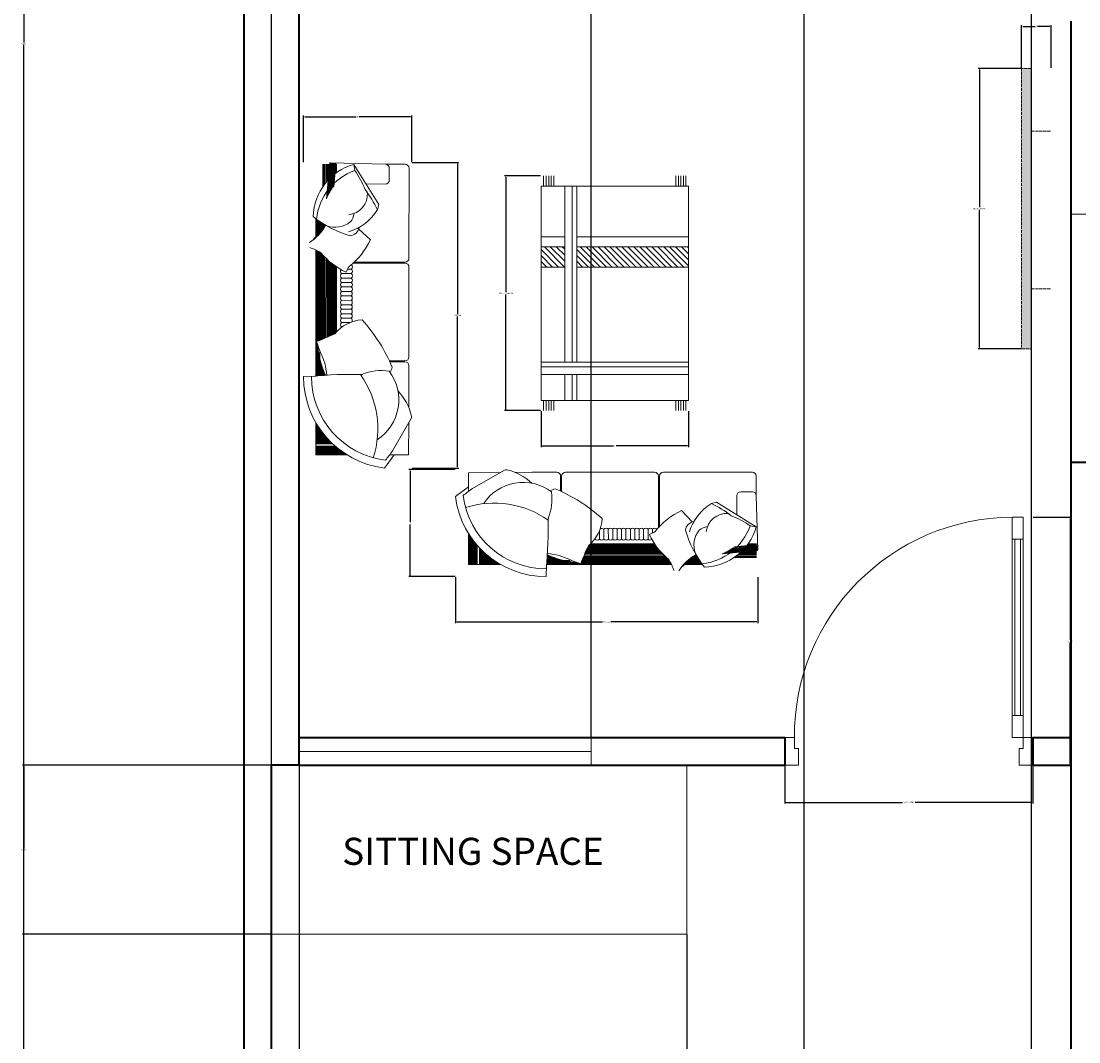
# Model space of a CAD drawing. Units: feet. Extents: x 1993 to 2298, y 2938 to 3641.
# Tile 5 of 11: x 1993 to 2147, y 3144 to 3293. Entities that reach past the tile are written whole.
import ezdxf

# ---------------------------------------------------------------- set-up
doc = ezdxf.new("R2010")
doc.units = ezdxf.units.FT
doc.linetypes.add('ACAD_ISO02W100', pattern=[15, 12, -3])
for name, color, linetype, lineweight in [('A-ANNO-DIMS', 2, 'Continuous', 18), ('A-AREA-IDEN', 7, 'Continuous', 18), ('A-DOOR', 3, 'Continuous', 18), ('A-FLOR-CASE', 8, 'Continuous', 18), ('A-GLAZ', 4, 'Continuous', 13), ('DWV_RED', 7, 'Continuous', 0), ('furniture', 8, 'Continuous', 18), ('SUNSHADES', 4, 'ACAD_ISO02W100', 13), ('WAL', 7, 'Continuous', 35)]:
    doc.layers.add(name, color=color, linetype=linetype, lineweight=lineweight)
doc.styles.get("Standard").update_dxf_attribs({"font": 'arial.ttf'})
doc.dimstyles.get("Standard").update_dxf_attribs({"dimtxt": 0.18, "dimasz": 0.18, "dimexe": 0.18, "dimexo": 0.0625, "dimgap": 0.09, "dimtad": 0, "dimtih": 1, "dimtoh": 1, "dimdec": 4, "dimzin": 0, "dimdsep": 46, "dimtxsty": 'Standard', "dimcen": 0.09, "dimadec": 0, "dimazin": 0, "dimtfac": 1, "dimtdec": 4, "dimtofl": 0, "dimtmove": 0, "dimatfit": 3, "dimfxl": 1, "dimtolj": 1, "dimtzin": 0, "dimarcsym": 0})

# ---------------------------------------------------------------- blocks, each defined once
blk = doc.blocks.new('A$C184E58E8')
for points in [[(825, 900), (825, 820), (865, 820), (865, 900)], [(825, 180), (825, 820), (865, 820), (865, 180)], [(835, 180), (835, 820), (855, 820), (855, 180)], [(825, 100), (825, 180), (865, 180), (865, 100)], [(35, 100), (35, 60), (50, 60), (50, 50), (50, 0), (0, 0), (0, 100)], [(865, 100), (900, 100), (900, 0), (850, 0), (850, 50), (850, 60), (865, 60)]]:
    blk.add_lwpolyline(points, close=True)
blk.add_arc((830, 105), 795, 90.3603, 180.3603)
blk = doc.blocks.new('A$C461A7772')
at = {"layer": 'DWV_RED'}
for p, q in [((15.4, 1855.9), (15.7, 1299.4)), ((161.8, 1880.4), (39.8, 1880.3)), ((137.4, 1856), (137.4, 1782.8)), ((161.8, 1880.4), (501.3, 1890.4)), ((203.1, 1631.1), (357.2, 1880)), ((350.1, 1842.2), (357.2, 1880)), ((463.7, 1880.6), (463.7, 1828.8)), ((463.7, 1880.6), (463.7, 1828.8)), ((463.7, 1880.6), (463.7, 1828.8)), ((467.9, 1887.3), (481.7, 1741.4)), ((469.8, 1880.6), (469.8, 1824.3)), ((469.8, 1880.6), (469.8, 1824.3)), ((471, 1880.6), (471, 1823.4)), ((472.2, 1880.6), (472.2, 1822.5)), ((472.8, 1887.7), (487.3, 1734.1)), ((474, 1880.6), (474.1, 1821.1)), ((475.9, 1880.6), (475.9, 1819.7)), ((477, 1888.1), (492.3, 1727.3)), ((478.3, 1880.6), (478.3, 1817.7)), ((480.7, 1880.6), (480.8, 1815.8)), ((481.3, 1888.5), (497.2, 1720.1)), ((483.8, 1880.6), (483.8, 1813.3)), ((484.9, 1888.9), (501.5, 1713.5)), ((486.8, 1880.6), (486.9, 1810.7)), ((488.6, 1889.2), (505.9, 1706.6)), ((490.5, 1880.6), (490.5, 1807.5)), ((491.6, 1889.5), (509.5, 1700.4)), ((494.1, 1880.6), (494.2, 1804.3)), ((494.6, 1889.8), (513.2, 1693.8)), ((497.1, 1890), (516.2, 1688.3)), ((498.4, 1880.6), (498.5, 1800.4)), ((499.5, 1890.3), (519.2, 1682.5)), ((501.3, 1890.4), (521.5, 1677.8)), ((502.7, 1880.6), (502.7, 1796.4)), ((503.1, 1890.6), (523.8, 1673)), ((504.3, 1890.7), (525.3, 1669.6)), ((505.6, 1890.8), (526.9, 1666.1)), ((505.6, 1890.8), (526.9, 1666.1)), ((507.6, 1880.6), (507.6, 1791.6)), ((512.4, 1880.6), (512.5, 1786.6)), ((517.9, 1880.6), (518, 1780.7)), ((523.4, 1880.6), (523.5, 1774.6)), ((530.8, 1766), (530.7, 1880.6)), ((538.1, 1880.6), (538.1, 1756.7)), ((543.6, 1880.6), (543.6, 1749.3)), ((549, 1880.6), (549.1, 1741.5)), ((281.9, 1758.5), (161.8, 1758.4)), ((210.9, 1599.5), (203.1, 1631.1)), ((538.3, 1507.5), (538.3, 1493.6)), ((543.7, 1510.8), (543.8, 1487.4)), ((549.2, 1514.2), (549.2, 1481.2)), ((554.1, 1517.3), (554.1, 1475.6)), ((559, 1520.4), (559, 1470.1)), ((563.2, 1523.2), (563.3, 1465.2)), ((567.5, 1526.1), (567.5, 1460.4)), ((571.2, 1528.5), (571.2, 1456.2)), ((574.8, 1531), (574.9, 1452.1)), ((577.9, 1533.1), (577.9, 1448.6)), ((580.9, 1535.3), (581, 1445.1)), ((583.4, 1537), (583.4, 1442.4)), ((585.8, 1538.7), (585.9, 1439.6)), ((587.6, 1540.1), (587.7, 1437.5)), ((589.5, 1541.4), (589.5, 1435.4)), ((590.7, 1542.3), (590.7, 1434)), ((591.9, 1543.2), (592, 1432.6)), ((591.9, 1543.2), (592, 1432.6)), ((254.5, 1413.5), (326.4, 1478.8)), ((530.2, 1502.8), (611.5, 1410.4)), ((530.9, 1501.9), (530.9, 1503.2)), ((543.8, 1313.9), (544.1, 800.3)), ((549.3, 1320), (549.6, 798.1)), ((554.2, 1325.6), (554.5, 796.1)), ((559.1, 1331.4), (559.4, 794.1)), ((563.3, 1335), (563.6, 792.4)), ((567.6, 1337.6), (567.9, 790.7)), ((571.3, 1339.7), (571.6, 789.3)), ((574.9, 1341.8), (575.2, 787.8)), ((578, 1343.5), (578.3, 786.7)), ((581, 1345.1), (581.3, 785.5)), ((583.5, 1346.4), (583.8, 784.6)), ((585.9, 1347.6), (586.2, 783.6)), ((587.7, 1348.5), (588, 782.9)), ((589.6, 1349.4), (590, 569.8)), ((590.8, 1349.9), (591.2, 569.7)), ((592, 1350.5), (592.4, 569.6)), ((15.7, 1244.5), (16, 688)), ((353.9, 1275.2), (40.1, 1275)), ((360.6, 1269.1), (40.1, 1268.9)), ((464, 1245.4), (464.2, 843.3)), ((470.1, 1249.6), (470.3, 836.5)), ((471.3, 1250.4), (471.5, 835.1)), ((472.5, 1251.3), (472.7, 833.7)), ((474.3, 1252.6), (474.6, 831.5)), ((476.2, 1253.9), (476.4, 830.3)), ((478.6, 1255.7), (478.8, 829.2)), ((481.1, 1257.5), (481.3, 828)), ((484.1, 1259.7), (484.3, 826.6)), ((487.1, 1262.1), (487.4, 825.2)), ((490.8, 1264.9), (491, 823.5)), ((494.5, 1267.8), (494.7, 821.8)), ((498.7, 1271.2), (499, 819.9)), ((503, 1274.8), (503.2, 818)), ((507.9, 1279), (508.1, 815.8)), ((512.8, 1283.3), (513, 813.6)), ((518.2, 1288.2), (518.5, 811.2)), ((523.7, 1293.4), (524, 808.8)), ((531.3, 805.7), (531, 1300.5)), ((538.4, 1308), (538.6, 802.6)), ((396.1, 1231.2), (372.5, 1231.2)), ((433.5, 1203.7), (372.5, 1203.6)), ((433.5, 1176.1), (372.5, 1176.1)), ((433.5, 1148.5), (372.5, 1148.5)), ((433.5, 1121), (372.6, 1120.9)), ((433.6, 1093.4), (372.6, 1093.4)), ((433.6, 1065.8), (372.6, 1065.8)), ((433.6, 1038.3), (372.6, 1038.2)), ((433.6, 1010.7), (372.6, 1010.7)), ((433.6, 983.1), (372.6, 983.1)), ((433.6, 955.6), (372.6, 955.5)), ((433.6, 928), (372.7, 928)), ((433.7, 900.4), (380.4, 900.4)), ((433.7, 872.9), (430.3, 872.9)), ((574.8, 643.5), (574.9, 722.5)), ((577.9, 641.4), (577.9, 726)), ((578.3, 756.8), (578.4, 570.9)), ((580.9, 639.3), (581, 729.4)), ((581.3, 764.5), (581.4, 570.6)), ((583.4, 637.6), (583.4, 732.2)), ((583.8, 770.6), (583.9, 570.4)), ((585.8, 635.8), (585.9, 735)), ((586.2, 776.7), (586.3, 570.2)), ((587.6, 634.5), (587.7, 737.1)), ((588, 781.3), (588.1, 570)), ((589.5, 633.2), (589.5, 739.1)), ((590.7, 632.3), (590.7, 740.5)), ((591.9, 631.4), (592, 741.9)), ((591.9, 631.4), (592, 741.9)), ((137.1, 663.7), (40.4, 663.6)), ((134.3, 657.6), (40.4, 657.5)), ((563.7, 661.6), (563.7, 572.1)), ((567.5, 648.5), (567.5, 714.2)), ((567.9, 678.4), (568, 571.7)), ((571.2, 646), (571.2, 718.4)), ((571.6, 694.7), (571.7, 571.4)), ((575.2, 713.6), (575.3, 571.1)), ((16, 633.1), (16.1, 479.1)), ((544.2, 601.6), (544.2, 573.6)), ((549.7, 616.5), (549.7, 573.2)), ((554.6, 630.8), (554.6, 572.8)), ((559.4, 646.5), (559.5, 572.4)), ((538.7, 587.9), (538.7, 574)), ((592.4, 569.6), (668.4, 567)), ((16.1, 479.1), (16.7, 374.1)), ((117.2, 107.3), (2.2, 306.3)), ((17.2, 280.4), (18.4, 81.6)), ((581.6, 264.1), (581.6, 209.5)), ((584, 268), (584, 209.5)), ((586.5, 272), (586.5, 209.5)), ((588.3, 275.1), (588.3, 209.5)), ((590.1, 278.2), (590.1, 209.5)), ((591.3, 280.3), (591.4, 209.5)), ((592.5, 282.4), (592.6, 81.5)), ((592.5, 282.4), (592.6, 209.5)), ((592.6, 197.3), (532.8, 197.3)), ((592.6, 199.2), (534.4, 199.1)), ((592.6, 201), (535.9, 201)), ((592.6, 202.2), (536.9, 202.2)), ((592.6, 203.4), (537.9, 203.4)), ((592.6, 203.4), (537.9, 203.4)), ((592.6, 209.5), (542.9, 209.5)), ((592.6, 209.5), (542.9, 209.5)), ((549.9, 218.5), (549.9, 209.5)), ((554.8, 224.9), (554.8, 209.5)), ((559.6, 231.5), (559.6, 209.5)), ((563.9, 237.5), (563.9, 209.5)), ((568.2, 243.6), (568.2, 209.5)), ((571.8, 249), (571.8, 209.5)), ((575.5, 254.5), (575.5, 209.5)), ((578.5, 259.3), (578.6, 209.5)), ((592.6, 135.1), (471.2, 135.1)), ((592.6, 149.8), (487.5, 149.7)), ((592.6, 155.3), (493.3, 155.2)), ((592.6, 160.8), (498.9, 160.7)), ((592.6, 165.6), (503.8, 165.6)), ((592.6, 170.5), (508.5, 170.5)), ((592.6, 174.8), (512.6, 174.7)), ((592.6, 179.1), (516.6, 179)), ((592.6, 182.7), (519.9, 182.7)), ((592.6, 186.4), (523.2, 186.3)), ((592.6, 189.4), (526, 189.4)), ((592.6, 192.5), (528.6, 192.4)), ((592.6, 194.9), (530.7, 194.9)), ((134.8, 82.3), (18.4, 81.6)), ((107.6, 81.2), (94.8, 81.2)), ((167.8, 0), (107.6, 81.2)), ((592.6, 81.5), (398.2, 81.4)), ((592.6, 81.5), (398.2, 81.4)), ((592.6, 82.7), (400.2, 82.6)), ((592.6, 83.9), (402.1, 83.8)), ((592.6, 85.7), (405, 85.6)), ((592.6, 87.6), (407.9, 87.5)), ((592.6, 90), (411.6, 89.9)), ((592.6, 92.4), (415.3, 92.4)), ((592.6, 95.5), (419.8, 95.4)), ((592.6, 98.5), (424.2, 98.5)), ((592.6, 102.2), (429.4, 102.1)), ((592.6, 105.9), (434.4, 105.8)), ((592.6, 110.1), (440.2, 110.1)), ((592.6, 114.4), (445.8, 114.3)), ((592.6, 119.3), (452.1, 119.2)), ((592.6, 124.2), (458.1, 124.1)), ((592.6, 129.7), (464.8, 129.6))]:
    blk.add_line(p, q, dxfattribs=at)
for centre, radius, start, end in [((39.8, 1855.9), 24.4, 90.02921, 180.02921), ((161.8, 1856), 24.4, 90.02921, 180.02921), ((843.8, 1506.7), 596.9, 145.79671, 158.68173), ((229.7, 1502), 360.9, 6.16007, 70.51656), ((261.8, 1545.8), 347.6, 1.73534, 74.06842), ((161.8, 1782.8), 24.4, 180.02921, 270.02921), ((813, 1312.9), 666.8, 141.97473, 154.54504), ((401.4, 1695.5), 128.4, 175.8739, 264.28215), ((483.3, 1768.4), 320.5, 211.79031, 252.92324), ((468.8, 1595.5), 115.5, 190.11899, 218.61362), ((473.2, 1642.9), 152.3, 231.63304, 289.73413), ((180.7, 2103.5), 695, 286.56402, 308.0684), ((385.8, 1500), 63, 188.56123, 263.66756), ((788.7, 1645.1), 294, 209.79721, 237.7813), ((656, 1597.1), 441.4, 204.57614, 232.37937), ((217.3, 1614), 443.5, 294.98785, 320.71747), ((700.5, 1116.5), 258, 105.83991, 122.83832), ((40.1, 1299.4), 24.4, 180.02921, 270.02921), ((40.1, 1244.5), 24.4, 90.02921, 180.02921), ((384.5, 1245), 18.3, 131.02639, 229.03203), ((241, 1150.7), 174.7, 20.53489, 33.62603), ((439.6, 1244.7), 24.4, 0.02921, 1.63163), ((384.5, 1217.4), 18.3, 131.02639, 229.03203), ((384.5, 1189.9), 18.3, 131.02639, 229.03203), ((421.5, 1217.4), 18.3, 311.02639, 36.47256), ((421.5, 1189.9), 18.3, 311.02639, 49.03203), ((384.5, 1162.3), 18.3, 131.02639, 229.03203), ((384.5, 1134.7), 18.3, 131.02639, 229.03203), ((384.5, 1107.2), 18.3, 131.02639, 229.03203), ((421.5, 1162.3), 18.3, 311.02639, 49.03203), ((421.6, 1134.7), 18.3, 311.02639, 49.03203), ((421.6, 1107.2), 18.3, 311.02639, 49.03203), ((384.6, 1079.6), 18.3, 131.02639, 229.03203), ((384.6, 1052), 18.3, 131.02639, 229.03203), ((421.6, 1079.6), 18.3, 311.02639, 49.03203), ((421.6, 1052), 18.3, 311.02639, 49.03203), ((384.6, 1024.5), 18.3, 131.02639, 229.03203), ((384.6, 996.9), 18.3, 131.02639, 229.03203), ((384.6, 969.3), 18.3, 131.02639, 229.03203), ((421.6, 1024.5), 18.3, 311.02639, 49.03203), ((421.6, 996.9), 18.3, 311.02639, 49.03203), ((421.6, 969.3), 18.3, 311.02639, 49.03203), ((1055, 236), 1012.6, 137.72097, 157.49241), ((291.2, 679.6), 238.1, 39.4723, 86.4925), ((384.6, 941.8), 18.3, 131.02639, 229.03203), ((384.6, 914.2), 18.3, 131.02639, 211.53959), ((421.7, 941.8), 18.3, 311.02639, 49.03203), ((421.7, 914.2), 18.3, 311.02639, 49.03203), ((421.7, 886.6), 18.3, 311.02639, 49.03203), ((1122.1, 2195.6), 1510.3, 244.63171, 249.31583), ((-23.3, 819.3), 607.8, 336.23493, 355.04803), ((4150.5, -654.9), 3841, 158.02042, 160.16759), ((40.4, 688), 24.4, 180.02921, 270.02921), ((40.4, 633.1), 24.4, 90.02921, 180.02921), ((373.7, 422.4), 294.9, 142.94543, 236.82049), ((326, 688.4), 216.4, 197.39352, 206.50126), ((184, 282.6), 320.8, 67.50059, 98.18972), ((1152.1, 499.1), 632.7, 166.36713, 173.11783), ((97.3, 566.7), 522.3, 277.09406, 0.02921), ((97.3, 566.7), 571.1, 277.09406, 0.02921), ((785.2, 243.2), 576.9, 144.37736, 198.14802), ((371.1, -1833.6), 2413.4, 84.09169, 91.66718), ((319.6, 249.8), 327.4, 136.03971, 167.46902), ((19.8, 316.5), 20.2, 167.46902, 210.00844), ((626.2, 446.5), 611.7, 213.68292, 220.60222)]:
    blk.add_arc(centre, radius, start, end, dxfattribs=at)
blk = doc.blocks.new('A$C1EBD441D')
at = {"layer": 'WAL', "xscale": -1, "rotation": 90}
blk.add_blockref('A$C461A7772', (1844.2, 649), dxfattribs=at)
blk = doc.blocks.new('A$C1BAF42B9')
at = {"layer": 'DWV_RED'}
h = blk.add_hatch(dxfattribs=at)
h.set_pattern_fill('ANSI31', color=256, scale=249.995738, angle=360, style=0)
h.set_pattern_definition([(45, (-691276.857, -155047.698), (-18.6440992, 18.6440992), [])])
h.paths.add_polyline_path([(699, 1024.4), (0, 1024.4), (0, 897.9), (699, 897.9)])
h.paths.add_polyline_path([(922.1, 1024.4), (774.5, 1024.4), (774.5, 897.9), (922.1, 897.9)])
for p, q in [((16.2, 1404.1), (16.2, 1467.4)), ((32, 1404.1), (32, 1467.4)), ((47.9, 1404.1), (47.9, 1467.4)), ((63.7, 1404.1), (63.7, 1467.4)), ((79.5, 1404.1), (79.5, 1467.4)), ((842.6, 1404.1), (842.6, 1467.4)), ((858.4, 1404.1), (858.4, 1467.4)), ((874.3, 1404.1), (874.3, 1467.4)), ((890.1, 1404.1), (890.1, 1467.4)), ((905.9, 1404.1), (905.9, 1467.4)), ((0, 1404.1), (922.1, 1404.1)), ((0, 63.3), (0, 1404.1)), ((699, 1404.1), (699, 302.2)), ((728, 1404.1), (728, 302.2)), ((774.5, 302.2), (774.5, 1404.1)), ((922.1, 1404.1), (922.1, 63.3)), ((0, 1087.7), (699, 1087.7)), ((774.5, 1087.7), (922.1, 1087.7)), ((0, 1024.4), (699, 1024.4)), ((774.5, 1024.4), (922.1, 1024.4)), ((0, 897.9), (699, 897.9)), ((774.5, 897.9), (922.1, 897.9)), ((922.1, 302.2), (0, 302.2)), ((922.1, 273.2), (0, 273.2)), ((922.1, 226.7), (0, 226.7)), ((699, 226.7), (699, 63.3)), ((728, 226.7), (728, 63.3)), ((774.5, 63.3), (774.5, 226.7)), ((922.1, 63.3), (0, 63.3)), ((16.2, 63.3), (16.2, 0)), ((32, 63.3), (32, 0)), ((47.9, 63.3), (47.9, 0)), ((63.7, 63.3), (63.7, 0)), ((79.5, 63.3), (79.5, 0)), ((842.6, 63.3), (842.6, 0)), ((858.4, 63.3), (858.4, 0)), ((874.3, 63.3), (874.3, 0)), ((890.1, 63.3), (890.1, 0)), ((905.9, 63.3), (905.9, 0))]:
    blk.add_line(p, q, dxfattribs=at)
blk = doc.blocks.new('A$C6E556493')
blk.add_hatch(color=256).paths.add_polyline_path([(1066.4, 112.5), (0, 112.5), (0, 75), (1066.4, 75)])
at = {"layer": 'SUNSHADES'}
for p, q in [((0, 75), (0, 112.5)), ((0, 112.5), (1066.4, 112.5)), ((1066.4, 112.5), (1066.4, 75)), ((1066.4, 75), (0, 75)), ((238.4, 75), (238.4, 0)), ((838.4, 75), (838.4, 0))]:
    blk.add_line(p, q, dxfattribs=at)
blk = doc.blocks.new('*D26')
at = {"layer": 'A-ANNO-DIMS', "color": 0, "lineweight": -2, "transparency": 16777216}
for p, q in [((2104.2, 3184.47), (2104.2, 3178.95)), ((2140.2, 3184.47), (2140.2, 3178.95)), ((2104.38, 3179.13), (2121.27, 3179.13)), ((2140.02, 3179.13), (2123.14, 3179.13))]:
    blk.add_line(p, q, dxfattribs=at)
at = {"layer": 'A-ANNO-DIMS', "color": 0, "transparency": 16777216}
for points in [[(2104.38, 3179.16), (2104.38, 3179.1), (2104.2, 3179.13)], [(2140.02, 3179.16), (2140.02, 3179.1), (2140.2, 3179.13)]]:
    blk.add_solid(points, dxfattribs=at)
at = {"layer": 'Defpoints', "color": 0, "transparency": 16777216}
for p in [(2104.2, 3184.53), (2140.2, 3184.53), (2140.2, 3179.13)]:
    blk.add_point(p, dxfattribs=at)
at = {"layer": 'A-ANNO-DIMS', "color": 0, "transparency": 16777216, "insert": (2122.2, 3179.13), "char_height": 0.18, "attachment_point": 5}
blk.add_mtext('\\A1;DOOR 36 TYP.', dxfattribs=at)
blk = doc.blocks.new('*D27')
at = {"layer": 'A-ANNO-DIMS', "color": 0, "lineweight": -2, "transparency": 16777216}
for p, q in [((2140.27, 3220.53), (2145.78, 3220.53)), ((2145.6, 3220.35), (2145.6, 3202.72)), ((2145.6, 3184.71), (2145.6, 3202.35)), ((2140.27, 3184.53), (2145.78, 3184.53))]:
    blk.add_line(p, q, dxfattribs=at)
at = {"layer": 'A-ANNO-DIMS', "color": 0, "transparency": 16777216}
for points in [[(2145.57, 3220.35), (2145.63, 3220.35), (2145.6, 3220.53)], [(2145.57, 3184.71), (2145.63, 3184.71), (2145.6, 3184.53)]]:
    blk.add_solid(points, dxfattribs=at)
at = {"layer": 'Defpoints', "color": 0, "transparency": 16777216}
for p in [(2140.2, 3220.53), (2145.6, 3220.53), (2140.2, 3184.53)]:
    blk.add_point(p, dxfattribs=at)
at = {"layer": 'A-ANNO-DIMS', "color": 0, "transparency": 16777216, "insert": (2145.6, 3202.53), "char_height": 0.18, "attachment_point": 5}
blk.add_mtext('\\A1;36 TYP.', dxfattribs=at)
blk = doc.blocks.new('*D42')
at = {"layer": 'A-ANNO-DIMS', "color": 0, "lineweight": -2, "transparency": 16777216}
for p, q in [((2050.15, 3272), (2056.91, 3272)), ((2056.73, 3271.82), (2056.73, 3250.02)), ((2056.73, 3227.85), (2056.73, 3249.65)), ((2050.15, 3227.67), (2056.91, 3227.67))]:
    blk.add_line(p, q, dxfattribs=at)
at = {"layer": 'A-ANNO-DIMS', "color": 0, "transparency": 16777216}
for points in [[(2056.7, 3271.82), (2056.76, 3271.82), (2056.73, 3272)], [(2056.7, 3227.85), (2056.76, 3227.85), (2056.73, 3227.67)]]:
    blk.add_solid(points, dxfattribs=at)
at = {"layer": 'Defpoints', "color": 0, "transparency": 16777216}
for p in [(2050.08, 3272), (2056.73, 3272), (2050.08, 3227.67)]:
    blk.add_point(p, dxfattribs=at)
at = {"layer": 'A-ANNO-DIMS', "color": 0, "transparency": 16777216, "insert": (2056.73, 3249.83), "char_height": 0.18, "attachment_point": 5}
blk.add_mtext('\\A1;SOFA 44', dxfattribs=at)
blk = doc.blocks.new('*D43')
at = {"layer": 'A-ANNO-DIMS', "color": 0, "lineweight": -2, "transparency": 16777216}
for p, q in [((2034.38, 3272.06), (2034.38, 3278.83)), ((2034.56, 3278.65), (2042.02, 3278.65)), ((2049.9, 3278.65), (2042.44, 3278.65)), ((2050.08, 3272.06), (2050.08, 3278.83))]:
    blk.add_line(p, q, dxfattribs=at)
at = {"layer": 'A-ANNO-DIMS', "color": 0, "transparency": 16777216}
for points in [[(2034.56, 3278.68), (2034.56, 3278.62), (2034.38, 3278.65)], [(2049.9, 3278.68), (2049.9, 3278.62), (2050.08, 3278.65)]]:
    blk.add_solid(points, dxfattribs=at)
at = {"layer": 'Defpoints', "color": 0, "transparency": 16777216}
for p in [(2034.38, 3278.65), (2034.38, 3272), (2050.08, 3272)]:
    blk.add_point(p, dxfattribs=at)
at = {"layer": 'A-ANNO-DIMS', "color": 0, "transparency": 16777216, "insert": (2042.23, 3278.65), "char_height": 0.18, "attachment_point": 5}
blk.add_mtext('\\A1;16', dxfattribs=at)
blk = doc.blocks.new('*D44')
at = {"layer": 'A-ANNO-DIMS', "color": 0, "lineweight": -2, "transparency": 16777216}
for p, q in [((2056.43, 3211.84), (2056.43, 3205.14)), ((2100.32, 3211.84), (2100.32, 3205.14)), ((2056.61, 3205.32), (2077.78, 3205.32)), ((2100.14, 3205.32), (2078.97, 3205.32))]:
    blk.add_line(p, q, dxfattribs=at)
at = {"layer": 'A-ANNO-DIMS', "color": 0, "transparency": 16777216}
for points in [[(2056.61, 3205.35), (2056.61, 3205.29), (2056.43, 3205.32)], [(2100.14, 3205.35), (2100.14, 3205.29), (2100.32, 3205.32)]]:
    blk.add_solid(points, dxfattribs=at)
at = {"layer": 'Defpoints', "color": 0, "transparency": 16777216}
for p in [(2056.43, 3211.9), (2100.32, 3211.9), (2056.43, 3205.32)]:
    blk.add_point(p, dxfattribs=at)
at = {"layer": 'A-ANNO-DIMS', "color": 0, "transparency": 16777216, "insert": (2078.38, 3205.32), "char_height": 0.18, "attachment_point": 5}
blk.add_mtext('\\A1;SOFA 44', dxfattribs=at)
blk = doc.blocks.new('*D45')
at = {"layer": 'A-ANNO-DIMS', "color": 0, "lineweight": -2, "transparency": 16777216}
for p, q in [((2056.37, 3227.45), (2049.67, 3227.45)), ((2049.85, 3227.27), (2049.85, 3219.86)), ((2049.85, 3212.08), (2049.85, 3219.49)), ((2056.37, 3211.9), (2049.67, 3211.9))]:
    blk.add_line(p, q, dxfattribs=at)
at = {"layer": 'A-ANNO-DIMS', "color": 0, "transparency": 16777216}
for points in [[(2049.82, 3227.27), (2049.88, 3227.27), (2049.85, 3227.45)], [(2049.82, 3212.08), (2049.88, 3212.08), (2049.85, 3211.9)]]:
    blk.add_solid(points, dxfattribs=at)
at = {"layer": 'Defpoints', "color": 0, "transparency": 16777216}
for p in [(2049.85, 3227.45), (2056.43, 3227.45), (2056.43, 3211.9)]:
    blk.add_point(p, dxfattribs=at)
at = {"layer": 'A-ANNO-DIMS', "color": 0, "transparency": 16777216, "insert": (2049.85, 3219.68), "char_height": 0.18, "attachment_point": 5}
blk.add_mtext('\\A1;16', dxfattribs=at)
blk = doc.blocks.new('*D46')
at = {"layer": 'A-ANNO-DIMS', "color": 0, "lineweight": -2, "transparency": 16777216}
for p, q in [((2068.79, 3270.06), (2063.56, 3270.06)), ((2063.74, 3269.88), (2063.74, 3253.21)), ((2063.74, 3236.18), (2063.74, 3252.84)), ((2068.79, 3236), (2063.56, 3236))]:
    blk.add_line(p, q, dxfattribs=at)
at = {"layer": 'A-ANNO-DIMS', "color": 0, "transparency": 16777216}
for points in [[(2063.71, 3269.88), (2063.77, 3269.88), (2063.74, 3270.06)], [(2063.71, 3236.18), (2063.77, 3236.18), (2063.74, 3236)]]:
    blk.add_solid(points, dxfattribs=at)
at = {"layer": 'Defpoints', "color": 0, "transparency": 16777216}
for p in [(2063.74, 3270.06), (2068.85, 3270.06), (2068.85, 3236)]:
    blk.add_point(p, dxfattribs=at)
at = {"layer": 'A-ANNO-DIMS', "color": 0, "transparency": 16777216, "insert": (2063.74, 3253.03), "char_height": 0.18, "attachment_point": 5}
blk.add_mtext('\\A1;COFFEE TABLE 34', dxfattribs=at)
blk = doc.blocks.new('*D47')
at = {"layer": 'A-ANNO-DIMS', "color": 0, "lineweight": -2, "transparency": 16777216}
for p, q in [((2068.85, 3235.93), (2068.85, 3230.71)), ((2090.26, 3235.93), (2090.26, 3230.71)), ((2069.03, 3230.89), (2079.35, 3230.89)), ((2090.08, 3230.89), (2079.76, 3230.89))]:
    blk.add_line(p, q, dxfattribs=at)
at = {"layer": 'A-ANNO-DIMS', "color": 0, "transparency": 16777216}
for points in [[(2069.03, 3230.92), (2069.03, 3230.86), (2068.85, 3230.89)], [(2090.08, 3230.92), (2090.08, 3230.86), (2090.26, 3230.89)]]:
    blk.add_solid(points, dxfattribs=at)
at = {"layer": 'Defpoints', "color": 0, "transparency": 16777216}
for p in [(2068.85, 3236), (2090.26, 3236), (2068.85, 3230.89)]:
    blk.add_point(p, dxfattribs=at)
at = {"layer": 'A-ANNO-DIMS', "color": 0, "transparency": 16777216, "insert": (2079.55, 3230.89), "char_height": 0.18, "attachment_point": 5}
blk.add_mtext('\\A1;21', dxfattribs=at)
blk = doc.blocks.new('*D48')
at = {"layer": 'A-ANNO-DIMS', "color": 0, "lineweight": -2, "transparency": 16777216}
for p, q in [((2138.51, 3285.68), (2132.28, 3285.68)), ((2132.46, 3285.5), (2132.46, 3265.51)), ((2132.46, 3245.16), (2132.46, 3265.15)), ((2138.51, 3244.98), (2132.28, 3244.98))]:
    blk.add_line(p, q, dxfattribs=at)
at = {"layer": 'A-ANNO-DIMS', "color": 0, "transparency": 16777216}
for points in [[(2132.43, 3285.5), (2132.49, 3285.5), (2132.46, 3285.68)], [(2132.43, 3245.16), (2132.49, 3245.16), (2132.46, 3244.98)]]:
    blk.add_solid(points, dxfattribs=at)
at = {"layer": 'Defpoints', "color": 0, "transparency": 16777216}
for p in [(2138.57, 3285.68), (2132.46, 3244.98), (2138.57, 3244.98)]:
    blk.add_point(p, dxfattribs=at)
at = {"layer": 'A-ANNO-DIMS', "color": 0, "transparency": 16777216, "insert": (2132.46, 3265.33), "char_height": 0.18, "attachment_point": 5}
blk.add_mtext('\\A1;MEDIA UNIT 41', dxfattribs=at)
blk = doc.blocks.new('*D49')
at = {"layer": 'A-ANNO-DIMS', "color": 0, "lineweight": -2, "transparency": 16777216}
for p, q in [((2138.57, 3285.74), (2138.57, 3291.96)), ((2138.75, 3291.78), (2140.56, 3291.78)), ((2142.68, 3291.78), (2140.87, 3291.78)), ((2142.86, 3285.74), (2142.86, 3291.96))]:
    blk.add_line(p, q, dxfattribs=at)
at = {"layer": 'A-ANNO-DIMS', "color": 0, "transparency": 16777216}
for points in [[(2138.75, 3291.81), (2138.75, 3291.75), (2138.57, 3291.78)], [(2142.68, 3291.81), (2142.68, 3291.75), (2142.86, 3291.78)]]:
    blk.add_solid(points, dxfattribs=at)
at = {"layer": 'Defpoints', "color": 0, "transparency": 16777216}
for p in [(2138.57, 3291.78), (2138.57, 3285.68), (2142.86, 3285.68)]:
    blk.add_point(p, dxfattribs=at)
at = {"layer": 'A-ANNO-DIMS', "color": 0, "transparency": 16777216, "insert": (2140.72, 3291.78), "char_height": 0.18, "attachment_point": 5}
blk.add_mtext('\\A1;4', dxfattribs=at)
blk = doc.blocks.new('*D56')
at = {"layer": 'A-ANNO-DIMS', "color": 0, "lineweight": -2, "transparency": 16777216}
for p, q in [((2025.7, 3608.53), (1993.61, 3608.53)), ((1993.79, 3608.35), (1993.79, 3289.45)), ((1993.79, 2970.18), (1993.79, 3289.08)), ((2029.7, 2970), (1993.61, 2970))]:
    blk.add_line(p, q, dxfattribs=at)
at = {"layer": 'A-ANNO-DIMS', "color": 0, "transparency": 16777216}
for points in [[(1993.76, 3608.35), (1993.82, 3608.35), (1993.79, 3608.53)], [(1993.76, 2970.18), (1993.82, 2970.18), (1993.79, 2970)]]:
    blk.add_solid(points, dxfattribs=at)
at = {"layer": 'Defpoints', "color": 0, "transparency": 16777216}
for p in [(1993.79, 3608.53), (2025.76, 3608.53), (2029.76, 2970)]:
    blk.add_point(p, dxfattribs=at)
at = {"layer": 'A-ANNO-DIMS', "color": 0, "transparency": 16777216, "insert": (1993.79, 3289.27), "char_height": 0.18, "attachment_point": 5}
blk.add_mtext('\\A1;638.5', dxfattribs=at)
blk = doc.blocks.new('*D59')
at = {"layer": 'A-ANNO-DIMS', "color": 0, "lineweight": -2, "transparency": 16777216}
for p, q in [((2140, 3048.6), (2140, 3640.68)), ((2140.18, 3640.5), (2144.79, 3640.5)), ((2149.82, 3640.5), (2145.21, 3640.5)), ((2150, 3048.6), (2150, 3640.68))]:
    blk.add_line(p, q, dxfattribs=at)
at = {"layer": 'A-ANNO-DIMS', "color": 0, "transparency": 16777216}
for points in [[(2140.18, 3640.53), (2140.18, 3640.47), (2140, 3640.5)], [(2149.82, 3640.53), (2149.82, 3640.47), (2150, 3640.5)]]:
    blk.add_solid(points, dxfattribs=at)
at = {"layer": 'Defpoints', "color": 0, "transparency": 16777216}
for p in [(2150, 3640.5), (2140, 3048.53), (2150, 3048.53)]:
    blk.add_point(p, dxfattribs=at)
at = {"layer": 'A-ANNO-DIMS', "color": 0, "transparency": 16777216, "insert": (2145, 3640.5), "char_height": 0.18, "attachment_point": 5}
blk.add_mtext('\\A1;10', dxfattribs=at)
blk = doc.blocks.new('*D67')
at = {"layer": 'A-ANNO-DIMS', "color": 0, "lineweight": -2, "transparency": 16777216}
for p, q in [((2033.76, 3428.47), (2033.76, 2937.86)), ((2106.96, 3428.47), (2106.96, 2937.86)), ((2033.94, 2938.03), (2070.03, 2938.03)), ((2106.78, 2938.03), (2070.68, 2938.03))]:
    blk.add_line(p, q, dxfattribs=at)
at = {"layer": 'A-ANNO-DIMS', "color": 0, "transparency": 16777216}
for points in [[(2033.94, 2938.07), (2033.94, 2938.01), (2033.76, 2938.03)], [(2106.78, 2938.07), (2106.78, 2938.01), (2106.96, 2938.03)]]:
    blk.add_solid(points, dxfattribs=at)
at = {"layer": 'Defpoints', "color": 0, "transparency": 16777216}
for p in [(2033.76, 3428.53), (2106.96, 3428.53), (2106.96, 2938.03)]:
    blk.add_point(p, dxfattribs=at)
at = {"layer": 'A-ANNO-DIMS', "color": 0, "transparency": 16777216, "insert": (2070.36, 2938.03), "char_height": 0.18, "attachment_point": 5}
blk.add_mtext('\\A1;73.2', dxfattribs=at)
blk = doc.blocks.new('*D71')
at = {"layer": 'A-ANNO-DIMS', "color": 0, "lineweight": -2, "transparency": 16777216}
for p, q in [((2029.76, 3159.94), (2029.76, 2937.86)), ((2090, 3159.94), (2090, 2937.86)), ((2029.94, 2938.03), (2059.49, 2938.03)), ((2089.82, 2938.03), (2060.27, 2938.03))]:
    blk.add_line(p, q, dxfattribs=at)
at = {"layer": 'A-ANNO-DIMS', "color": 0, "transparency": 16777216}
for points in [[(2029.94, 2938.07), (2029.94, 2938.01), (2029.76, 2938.03)], [(2089.82, 2938.07), (2089.82, 2938.01), (2090, 2938.03)]]:
    blk.add_solid(points, dxfattribs=at)
at = {"layer": 'Defpoints', "color": 0, "transparency": 16777216}
for p in [(2029.76, 3160), (2090, 3160), (2090, 2938.03)]:
    blk.add_point(p, dxfattribs=at)
at = {"layer": 'A-ANNO-DIMS', "color": 0, "transparency": 16777216, "insert": (2059.88, 2938.03), "char_height": 0.18, "attachment_point": 5}
blk.add_mtext('\\A1;60.24', dxfattribs=at)
blk = doc.blocks.new('*D72')
at = {"layer": 'A-ANNO-DIMS', "color": 0, "lineweight": -2, "transparency": 16777216}
for p, q in [((2029.7, 3184.53), (1993.61, 3184.53)), ((1993.79, 3184.35), (1993.79, 3172.45)), ((1993.79, 3160.18), (1993.79, 3172.08)), ((2029.7, 3160), (1993.61, 3160))]:
    blk.add_line(p, q, dxfattribs=at)
at = {"layer": 'A-ANNO-DIMS', "color": 0, "transparency": 16777216}
for points in [[(1993.76, 3184.35), (1993.82, 3184.35), (1993.79, 3184.53)], [(1993.76, 3160.18), (1993.82, 3160.18), (1993.79, 3160)]]:
    blk.add_solid(points, dxfattribs=at)
at = {"layer": 'Defpoints', "color": 0, "transparency": 16777216}
for p in [(1993.79, 3184.53), (2029.76, 3184.53), (2029.76, 3160)]:
    blk.add_point(p, dxfattribs=at)
at = {"layer": 'A-ANNO-DIMS', "color": 0, "transparency": 16777216, "insert": (1993.79, 3172.27), "char_height": 0.18, "attachment_point": 5}
blk.add_mtext('\\A1;24.534', dxfattribs=at)
blk = doc.blocks.new('*D75')
at = {"layer": 'A-ANNO-DIMS', "color": 0, "lineweight": -2, "transparency": 16777216}
for p, q in [((2029.76, 3008.6), (2029.76, 3640.68)), ((2029.94, 3640.5), (2084.42, 3640.5)), ((2139.82, 3640.5), (2085.33, 3640.5)), ((2140, 3008.6), (2140, 3640.68))]:
    blk.add_line(p, q, dxfattribs=at)
at = {"layer": 'A-ANNO-DIMS', "color": 0, "transparency": 16777216}
for points in [[(2029.94, 3640.53), (2029.94, 3640.47), (2029.76, 3640.5)], [(2139.82, 3640.53), (2139.82, 3640.47), (2140, 3640.5)]]:
    blk.add_solid(points, dxfattribs=at)
at = {"layer": 'Defpoints', "color": 0, "transparency": 16777216}
for p in [(2140, 3640.5), (2029.76, 3008.53), (2140, 3008.53)]:
    blk.add_point(p, dxfattribs=at)
at = {"layer": 'A-ANNO-DIMS', "color": 0, "transparency": 16777216, "insert": (2084.88, 3640.5), "char_height": 0.18, "attachment_point": 5}
blk.add_mtext('\\A1;110.24', dxfattribs=at)
blk = doc.blocks.new('*D76')
at = {"layer": 'A-ANNO-DIMS', "color": 0, "lineweight": -2, "transparency": 16777216}
for p, q in [((2033.76, 3188.6), (2033.76, 3640.68)), ((2033.94, 3640.5), (2054.54, 3640.5)), ((2075.93, 3640.5), (2055.33, 3640.5)), ((2076.11, 3188.6), (2076.11, 3640.68))]:
    blk.add_line(p, q, dxfattribs=at)
at = {"layer": 'A-ANNO-DIMS', "color": 0, "transparency": 16777216}
for points in [[(2033.94, 3640.53), (2033.94, 3640.47), (2033.76, 3640.5)], [(2075.93, 3640.53), (2075.93, 3640.47), (2076.11, 3640.5)]]:
    blk.add_solid(points, dxfattribs=at)
at = {"layer": 'Defpoints', "color": 0, "transparency": 16777216}
for p in [(2076.11, 3640.5), (2033.76, 3188.53), (2076.11, 3188.53)]:
    blk.add_point(p, dxfattribs=at)
at = {"layer": 'A-ANNO-DIMS', "color": 0, "transparency": 16777216, "insert": (2054.93, 3640.5), "char_height": 0.18, "attachment_point": 5}
blk.add_mtext('\\A1;42.35', dxfattribs=at)

msp = doc.modelspace()

# ---------------------------------------------------------------- linework, layer by layer
at = {"layer": 'A-FLOR-CASE'}
for p, q in [((2090, 3184.5338), (2090, 3160)), ((2090, 3160), (2029.7583, 3160))]:
    msp.add_line(p, q, dxfattribs=at)
at = {"layer": 'A-GLAZ'}
for p, q in [((2145.7583, 3264.5338), (2149.7583, 3264.5338)), ((2076.1089, 3188.5338), (2076.1089, 3184.5338)), ((2033.7583, 3186.5338), (2076.1089, 3186.5338))]:
    msp.add_line(p, q, dxfattribs=at)
at = {"layer": 'WAL'}
for p, q in [((2025.7583, 3008.5338), (2025.7583, 3608.5338)), ((2033.7583, 3184.5338), (2033.7583, 3600.5338)), ((2145.7583, 3084.5338), (2145.7583, 3292.5338)), ((2145.7583, 3228.5338), (2257.7583, 3228.5338)), ((2033.7583, 3188.5338), (2104.203, 3188.5338)), ((2104.203, 3188.5338), (2104.203, 3184.5338)), ((2140.203, 3188.5338), (2140.203, 3184.5338)), ((2140.203, 3188.5338), (2145.7583, 3188.5338)), ((2033.7583, 3184.5338), (2029.7583, 3184.5338)), ((2029.7583, 3008.5338), (2029.7583, 3184.5338)), ((2033.7583, 3184.5338), (2104.203, 3184.5338)), ((2140.203, 3184.5338), (2145.7583, 3184.5338))]:
    msp.add_line(p, q, dxfattribs=at)

# ---------------------------------------------------------------- block references
at = {"layer": 'A-DOOR', "xscale": 0.0400000004772489, "yscale": 0.0400000004772489, "zscale": 0.0400000004772489}
msp.add_blockref('A$C184E58E8', (2104.203, 3184.5338), dxfattribs=at)
at = {"layer": 'furniture', "xscale": -0.0381644559206992, "yscale": 0.0381644559206992, "zscale": 0.0381644559206992, "rotation": 90.00003968500015}
msp.add_blockref('A$C6E556493', (2142.8623, 3285.6769), dxfattribs=at)
at = {"layer": 'furniture'}
for name, p, xscale, yscale, zscale in [('A$C461A7772', (2050.0574, 3227.6653), -0.0234468844652987, 0.0234468844652987, 0.0234468844652987), ('A$C1BAF42B9', (2090.2563, 3235.9954), -0.0232133139471856, 0.0232133139471856, 0.0232133139471856), ('A$C1EBD441D', (2099.2407, 3212.3549), -0.0232133139471856, 0.0232133139471856, 0.0232133139471856)]:
    msp.add_blockref(name, p, dxfattribs=dict(at, xscale=xscale, yscale=yscale, zscale=zscale))

# ---------------------------------------------------------------- texts
at = {"layer": 'A-AREA-IDEN'}
msp.add_text('SITTING SPACE', height=3.928054, dxfattribs=at).set_placement((2040, 3170.067))

# ---------------------------------------------------------------- dimensions: what is measured, and where the dimension line sits
at = {"layer": 'A-ANNO-DIMS'}
for base, p1, p2, override, picture, middle in [((2140, 3640.4988), (2029.7583, 3008.5338), (2140, 3008.5338), {"dimdec": 2, "dimlfac": 1, "dimrnd": 0, "dimzin": 0, "dimdsep": 46, "dimlunit": 2}, '*D75', (2084.8792, 3640.4988)), ((2076.1089, 3640.4988), (2033.7583, 3188.5338), (2076.1089, 3188.5338), {"dimdec": 2, "dimlfac": 1, "dimrnd": 0, "dimzin": 0, "dimdsep": 46, "dimlunit": 2}, '*D76', (2054.9336, 3640.4988)), ((2150, 3640.4988), (2140, 3048.5338), (2150, 3048.5338), {"dimdec": 0, "dimlfac": 1, "dimrnd": 0, "dimzin": 0, "dimdsep": 46, "dimlunit": 2}, '*D59', (2145, 3640.4988)), ((2106.9556, 2938.035), (2033.7583, 3428.5338), (2106.9556, 3428.5338), {"dimdec": 1, "dimlfac": 1, "dimrnd": 0, "dimzin": 0, "dimdsep": 46, "dimlunit": 2}, '*D67', (2070.357, 2938.035)), ((2090, 2938.035), (2029.7583, 3160), (2090, 3160), {"dimdec": 2, "dimlfac": 1, "dimrnd": 0, "dimzin": 0, "dimdsep": 46, "dimlunit": 2}, '*D71', (2059.8792, 2938.035))]:
    dim = msp.add_linear_dim(base=base, p1=p1, p2=p2, dimstyle='Standard', override=override, dxfattribs=at)
    dim.commit()
    dim.dimension.update_dxf_attribs({"geometry": picture, "text_midpoint": middle})
for base, p1, p2, angle, override, picture, middle in [((1993.7933, 3608.5338), (2029.7583, 2970), (2025.7583, 3608.5338), 90, {"dimdec": 1, "dimlfac": 1, "dimrnd": 0, "dimzin": 0, "dimdsep": 46, "dimlunit": 2}, '*D56', (1993.7933, 3289.2669)), ((2138.5688, 3291.7817), (2142.8623, 3285.6769), (2138.5688, 3285.6769), 180.00004, {"dimdec": 0, "dimlfac": 1, "dimrnd": 0, "dimzin": 0, "dimdsep": 46, "dimlunit": 2}, '*D49', (2140.7156, 3291.7817)), ((2034.3832, 3278.6499), (2050.0832, 3271.9997), (2034.3832, 3271.9997), 180, {"dimdec": 0, "dimlfac": 1, "dimrnd": 0, "dimzin": 0, "dimdsep": 46, "dimlunit": 2}, '*D43', (2042.2332, 3278.6499)), ((2068.851, 3230.8859), (2090.2562, 3235.9954), (2068.851, 3235.9954), 180, {"dimdec": 0, "dimlfac": 1, "dimrnd": 0, "dimzin": 0, "dimdsep": 46, "dimlunit": 2}, '*D47', (2079.5536, 3230.8859)), ((2049.8468, 3227.447), (2056.4307, 3211.9034), (2056.4307, 3227.447), 90, {"dimdec": 0, "dimlfac": 1, "dimrnd": 0, "dimzin": 0, "dimdsep": 46, "dimlunit": 2}, '*D45', (2049.8468, 3219.6752)), ((1993.7933, 3184.5338), (2029.7583, 3160), (2029.7583, 3184.5338), 90, {"dimdec": 3, "dimlfac": 1, "dimrnd": 0, "dimzin": 0, "dimdsep": 46, "dimlunit": 2}, '*D72', (1993.7933, 3172.2669))]:
    dim = msp.add_linear_dim(base=base, p1=p1, p2=p2, angle=angle, dimstyle='Standard', override=override, dxfattribs=at)
    dim.commit()
    dim.dimension.update_dxf_attribs({"geometry": picture, "text_midpoint": middle})
for base, p1, p2, angle, text, picture, middle in [((2132.464, 3244.9776), (2138.5688, 3285.6769), (2138.5689, 3244.9776), 270.00004, 'MEDIA UNIT <>', '*D48', (2132.464, 3265.3272)), ((2056.7334, 3271.9997), (2050.0832, 3227.6653), (2050.0832, 3271.9997), 90, 'SOFA <>', '*D42', (2056.7334, 3249.8325)), ((2063.7415, 3270.0588), (2068.851, 3235.9954), (2068.851, 3270.0588), 90, 'COFFEE TABLE <>', '*D46', (2063.7415, 3253.0271)), ((2145.603, 3220.5338), (2140.203, 3184.5338), (2140.203, 3220.5338), 90, '<> TYP.', '*D27', (2145.603, 3202.5338)), ((2056.4307, 3205.3195), (2100.3235, 3211.9034), (2056.4307, 3211.9034), 180, 'SOFA <>', '*D44', (2078.3771, 3205.3195))]:
    dim = msp.add_linear_dim(base=base, p1=p1, p2=p2, angle=angle, text=text, dimstyle='Standard', override={"dimdec": 0, "dimlfac": 1, "dimrnd": 0, "dimzin": 0, "dimdsep": 46, "dimlunit": 2}, dxfattribs=at)
    dim.commit()
    dim.dimension.update_dxf_attribs({"geometry": picture, "text_midpoint": middle})
dim = msp.add_linear_dim(base=(2140.203, 3179.1338), p1=(2104.203, 3184.5338), p2=(2140.203, 3184.5338), text='DOOR <> TYP.', dimstyle='Standard', override={"dimdec": 0, "dimlfac": 1, "dimrnd": 0, "dimzin": 0, "dimdsep": 46, "dimlunit": 2}, dxfattribs=at)
dim.commit()
dim.dimension.update_dxf_attribs({"geometry": '*D26', "text_midpoint": (2122.203, 3179.1338)})

doc.saveas('drawing.dxf')
